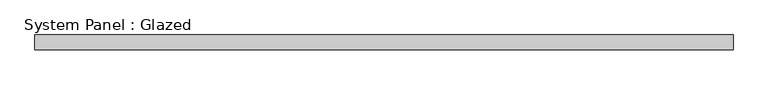
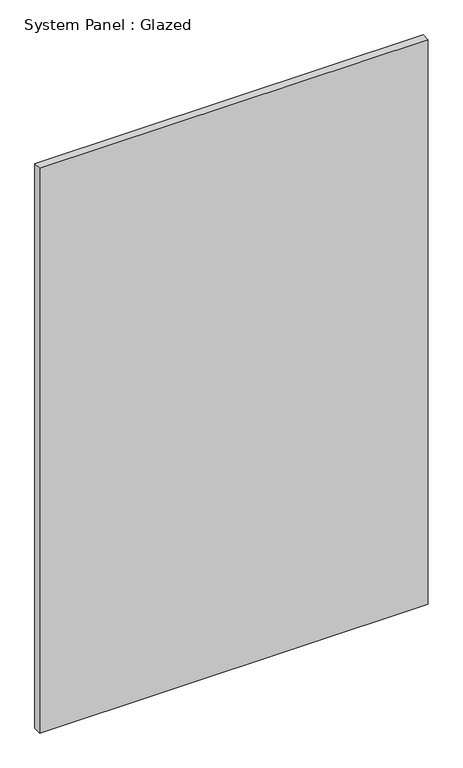
"""IFC4 building model written with IfcOpenShell, lengths in millimetres: plate geometry, System Panel : Glazed."""

from ifc_helpers import new_model, si_unit, origin, origin_with_axes, place, context, project, spatial, polyline, outline, extrude, source, transform, mapped, element, save


def system_panel_glazed_c585f582(model_context):
    return source(origin(), model_context, "Body", "SweptSolid", [
        extrude(outline(polyline([(600.075, 19.05), (-600.075, 19.05), (-600.075, 44.45), (600.075, 44.45), (600.075, 19.05)])), origin_with_axes(), (0.0, 0.0, 1.0), 1843.8332834),
    ])


if __name__ == "__main__":
    model = new_model("IFC4")
    model_context = context("Model", 3, world=origin())
    ifc_project = project(units=[si_unit("LENGTHUNIT", "METRE", prefix="MILLI")], contexts=[model_context])
    site = spatial("IfcSite", under=ifc_project)
    building = spatial("IfcBuilding", under=site)
    placement = place(None, origin())
    system_panel_glazed_shape = system_panel_glazed_c585f582(model_context)
    element("IfcPlate", 1, ObjectType="System Panel : Glazed", at=placement, inside=building, context=model_context, shape_type="MappedRepresentation", body=[
        mapped(system_panel_glazed_shape, transform((0.0, 0.0, 0.0), x_axis=(1.0, 0.0, 0.0), y_axis=(0.0, 1.0, 0.0), z_axis=(0.0, 0.0, 1.0))),
    ])
    save(model, "model.ifc")

# Revit data of these elements
# Type "System Panel : Glazed"
#   Construction Type Id = "GSP4R"
#   Analytic Construction = "1/8 in Pilkington single glazing"
#   Visual Light Transmittance = 0.9
#   Solar Heat Gain Coefficient = 0.86
#   Heat Transfer Coefficient (U) = 1.18115 BTU/(h·ft²·°F)
#   Define Thermal Properties by = 1
# Element 1 (IfcPlate, "System Panel : Glazed")
#   Materials on its faces: "Glass"
# Materials
#   "Glass": class "Glass", colour RGB 0 128 192, transparency 0.75, Description = "Soda Lime Glass", Cost = 0
